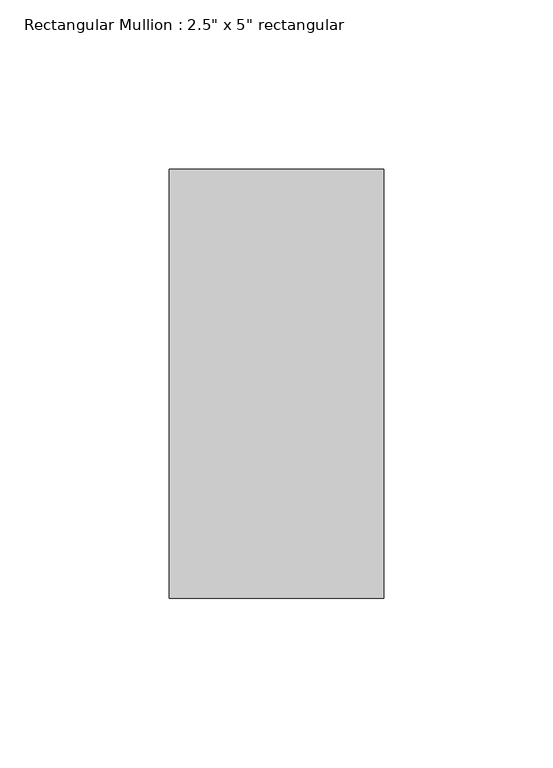
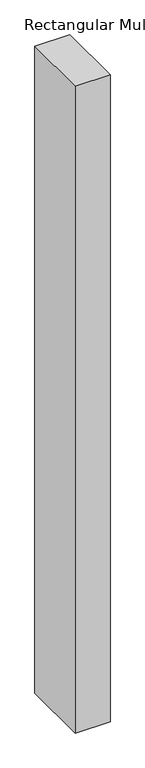
"""IFC4 building model written with IfcOpenShell, lengths in millimetres: member geometry."""

from ifc_helpers import new_model, si_unit, frame, origin, place, context, project, spatial, polyline, outline, extrude, source, transform, mapped, element, save


def member_71eb4692(model_context):
    return source(origin(), model_context, "Body", "SweptSolid", [
        extrude(outline(polyline([(0.0, 63.5), (0.0, -63.5), (-63.5, -63.5), (-63.5, 63.5), (0.0, 63.5)])), frame((0.0, 0.0, -1244.6), z_axis=(0.0, 0.0, 1.0), x_axis=(1.0, 0.0, 0.0)), (0.0, 0.0, 1.0), 1244.6),
    ])


if __name__ == "__main__":
    model = new_model("IFC4")
    model_context = context("Model", 3, world=origin())
    ifc_project = project(units=[si_unit("LENGTHUNIT", "METRE", prefix="MILLI")], contexts=[model_context])
    site = spatial("IfcSite", under=ifc_project)
    building = spatial("IfcBuilding", under=site)
    placement = place(None, origin())
    member_shape = member_71eb4692(model_context)
    element("IfcMember", 1, ObjectType="Rectangular Mullion : 2.5\" x 5\" rectangular", at=placement, inside=building, context=model_context, shape_type="MappedRepresentation", body=[
        mapped(member_shape, transform((0.0, 0.0, 0.0), x_axis=(1.0, 0.0, 0.0), y_axis=(0.0, 1.0, 0.0), z_axis=(0.0, 0.0, 1.0))),
    ])
    save(model, "model.ifc")

# Revit data of these elements
# Type "Rectangular Mullion : 2.5\" x 5\" rectangular"
#   built-in parameter 1007304 = 0.416667 (stored number, unit not read)
#   built-in parameter 1007301 = 0.104167 (stored number, unit not read)
#   built-in parameter 1007300 = 0.104167 (stored number, unit not read)
# Element 1 (IfcMember, "Rectangular Mullion : 2.5\" x 5\" rectangular")
#   Materials on its faces: "Aluminum"
# Materials
#   "Aluminum": class "Metal", colour RGB 247 247 247, transparency 0, Description = "Aluminum 6061", Cost = 0
